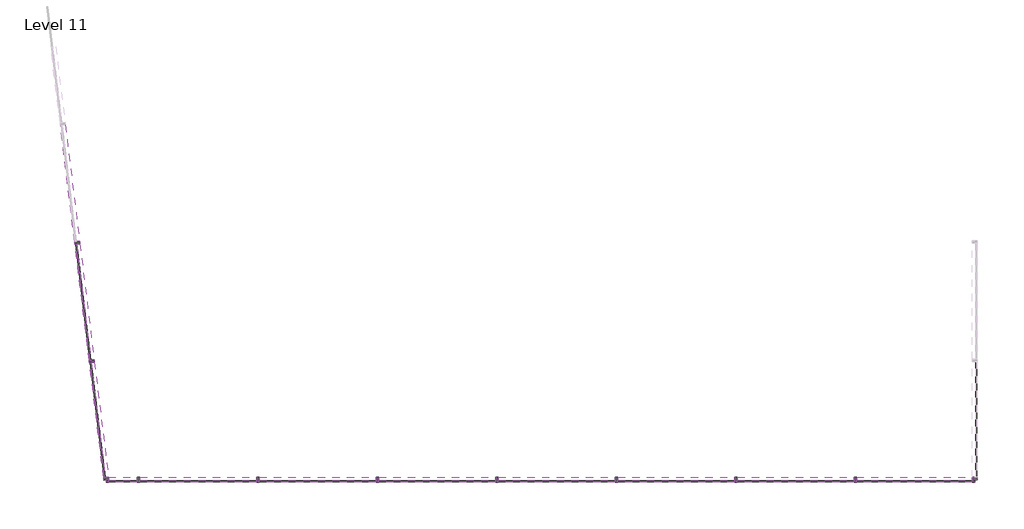
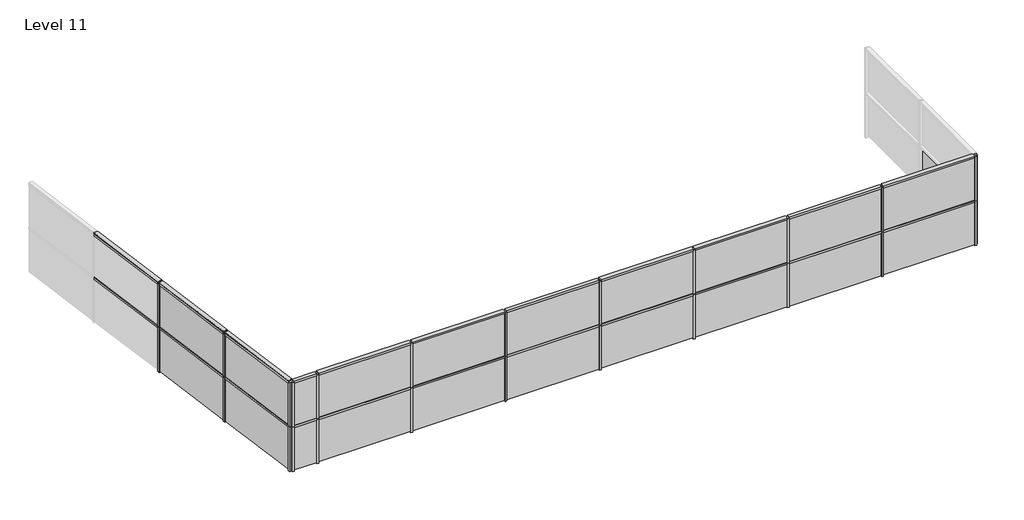
# One storey, part 1 of 2: 60 members, 25 plates.
"""IFC4 building model written with IfcOpenShell, lengths in millimetres."""

from ifc_helpers import new_model, si_unit, origin, place, context, project, spatial, transform, mapped, element, save
from components import member_daa7a266, member_82905deb, member_19d0a4ec, member_8cef0660, member_db480205, member_4491d118, member_0c11e56c, system_panel_glazed_37f15d2e, system_panel_glazed_3620f98e, system_panel_glazed_e46d4b42, system_panel_glazed_2a6c68b7, system_panel_glazed_9d0e0944

model = new_model("IFC4")

# Units and contexts
model_context = context("Model", 3, world=origin())
ifc_project = project(units=[si_unit("LENGTHUNIT", "METRE", prefix="MILLI")], contexts=[model_context])

# Site, building, storey
site = spatial("IfcSite", under=ifc_project)
building = spatial("IfcBuilding", under=site)
storey = spatial("IfcBuildingStorey", under=building, Name="Level 11", Elevation=30480.0)

# Members
placement = place(None, origin())
member_shape = member_daa7a266(model_context)
element("IfcMember", 1, ObjectType="Rectangular Mullion : 2.5\" x 5\" rectangular", at=placement, inside=storey, context=model_context, shape_type="MappedRepresentation", body=[
    mapped(member_shape, transform((-8260.4765148, -6916.1096898, 33528.0), x_axis=(0.0, 0.0, 1.0), y_axis=(-0.9925461516413222, -0.12186934340514587, 0.0), z_axis=(0.12186934340514587, -0.9925461516413222, 0.0))),
])
member_2_shape = member_82905deb(model_context)
element("IfcMember", 2, ObjectType="Rectangular Mullion : 2.5\" x 5\" rectangular", at=placement, inside=storey, context=model_context, shape_type="MappedRepresentation", body=[
    mapped(member_2_shape, transform((-8624.1955702, -3953.8557, 33528.0), x_axis=(-0.1218693434051459, 0.9925461516413222, 0.0), y_axis=(-0.9925461516413222, -0.1218693434051459, 0.0), z_axis=(0.0, 0.0, 1.0))),
])
element("IfcMember", 3, ObjectType="Rectangular Mullion : 2.5\" x 5\" rectangular", at=placement, inside=storey, context=model_context, shape_type="MappedRepresentation", body=[
    mapped(member_2_shape, transform((-8995.6533289, -928.5750297, 33528.0), x_axis=(-0.1218693434051459, 0.9925461516413222, 0.0), y_axis=(-0.9925461516413222, -0.1218693434051459, 0.0), z_axis=(0.0, 0.0, 1.0))),
])
member_3_shape = member_19d0a4ec(model_context)
element("IfcMember", 4, ObjectType="Rectangular Mullion : 2.5\" x 5\" rectangular", at=placement, inside=storey, context=model_context, shape_type="MappedRepresentation", body=[
    mapped(member_3_shape, transform((-8260.4765148, -6916.1096898, 32004.0), x_axis=(0.0, 0.0, 1.0), y_axis=(-0.9925461516413222, -0.12186934340514567, 0.0), z_axis=(0.12186934340514567, -0.9925461516413222, 0.0))),
])
element("IfcMember", 5, ObjectType="Rectangular Mullion : 2.5\" x 5\" rectangular", at=placement, inside=storey, context=model_context, shape_type="MappedRepresentation", body=[
    mapped(member_3_shape, transform((-8260.4765148, -6916.1096898, 32004.0), x_axis=(0.0, 0.0, 1.0), y_axis=(-0.9925461516413222, -0.12186934340514594, 0.0), z_axis=(0.12186934340514592, -0.9925461516413221, 0.0))),
])
element("IfcMember", 6, ObjectType="Rectangular Mullion : 2.5\" x 5\" rectangular", at=placement, inside=storey, context=model_context, shape_type="MappedRepresentation", body=[
    mapped(member_3_shape, transform((-8260.4765148, -6916.1096898, 33528.0), x_axis=(0.0, 0.0, 1.0), y_axis=(-0.9925461516413222, -0.12186934340514585, 0.0), z_axis=(0.12186934340514584, -0.9925461516413221, 0.0))),
])
element("IfcMember", 7, ObjectType="Rectangular Mullion : 2.5\" x 5\" rectangular", at=placement, inside=storey, context=model_context, shape_type="MappedRepresentation", body=[
    mapped(member_3_shape, transform((13839.0156363, -6979.1363705, 32004.0), x_axis=(0.0, 0.0, 1.0), y_axis=(0.0, -1.0, 0.0), z_axis=(1.0, 0.0, 0.0))),
])
element("IfcMember", 8, ObjectType="Rectangular Mullion : 2.5\" x 5\" rectangular", at=placement, inside=storey, context=model_context, shape_type="MappedRepresentation", body=[
    mapped(member_3_shape, transform((13839.0156363, -6979.1363705, 33528.0), x_axis=(0.0, 0.0, 1.0), y_axis=(0.0, -1.0, 0.0), z_axis=(1.0, 0.0, 0.0))),
])
member_4_shape = member_8cef0660(model_context)
element("IfcMember", 9, ObjectType="Rectangular Mullion : 2.5\" x 5\" rectangular", at=placement, inside=storey, context=model_context, shape_type="MappedRepresentation", body=[
    mapped(member_4_shape, transform((-8628.0649219, -3922.3423596, 32004.0), x_axis=(0.0, 0.0, 1.0), y_axis=(-0.9925461516413222, -0.12186934340514595, 0.0), z_axis=(0.12186934340514595, -0.9925461516413222, 0.0))),
])
element("IfcMember", 10, ObjectType="Rectangular Mullion : 2.5\" x 5\" rectangular", at=placement, inside=storey, context=model_context, shape_type="MappedRepresentation", body=[
    mapped(member_4_shape, transform((-8999.5226806, -897.0616894, 32004.0), x_axis=(0.0, 0.0, 1.0), y_axis=(-0.9925461516413222, -0.12186934340514599, 0.0), z_axis=(0.12186934340514599, -0.9925461516413222, 0.0))),
])
element("IfcMember", 11, ObjectType="Rectangular Mullion : 2.5\" x 5\" rectangular", at=placement, inside=storey, context=model_context, shape_type="MappedRepresentation", body=[
    mapped(member_4_shape, transform((-8628.0649219, -3922.3423596, 32004.0), x_axis=(0.0, 0.0, 1.0), y_axis=(-0.9925461516413222, -0.12186934340514607, 0.0), z_axis=(0.12186934340514607, -0.9925461516413222, 0.0))),
])
element("IfcMember", 12, ObjectType="Rectangular Mullion : 2.5\" x 5\" rectangular", at=placement, inside=storey, context=model_context, shape_type="MappedRepresentation", body=[
    mapped(member_4_shape, transform((-8999.5226806, -897.0616894, 32004.0), x_axis=(0.0, 0.0, 1.0), y_axis=(-0.9925461516413222, -0.12186934340514592, 0.0), z_axis=(0.12186934340514592, -0.9925461516413222, 0.0))),
])
element("IfcMember", 13, ObjectType="Rectangular Mullion : 2.5\" x 5\" rectangular", at=placement, inside=storey, context=model_context, shape_type="MappedRepresentation", body=[
    mapped(member_4_shape, transform((-8628.0649219, -3922.3423596, 33528.0), x_axis=(0.0, 0.0, 1.0), y_axis=(-0.9925461516413222, -0.1218693434051457, 0.0), z_axis=(0.1218693434051457, -0.9925461516413222, 0.0))),
])
element("IfcMember", 14, ObjectType="Rectangular Mullion : 2.5\" x 5\" rectangular", at=placement, inside=storey, context=model_context, shape_type="MappedRepresentation", body=[
    mapped(member_4_shape, transform((-8999.5226806, -897.0616894, 33528.0), x_axis=(0.0, 0.0, 1.0), y_axis=(-0.9925461516413222, -0.12186934340514595, 0.0), z_axis=(0.12186934340514595, -0.9925461516413222, 0.0))),
])
element("IfcMember", 15, ObjectType="Rectangular Mullion : 2.5\" x 5\" rectangular", at=placement, inside=storey, context=model_context, shape_type="MappedRepresentation", body=[
    mapped(member_4_shape, transform((10822.765636, -6979.1363705, 32004.0), x_axis=(0.0, 0.0, 1.0), y_axis=(0.0, -1.0, 0.0), z_axis=(1.0, 0.0, 0.0))),
])
element("IfcMember", 16, ObjectType="Rectangular Mullion : 2.5\" x 5\" rectangular", at=placement, inside=storey, context=model_context, shape_type="MappedRepresentation", body=[
    mapped(member_4_shape, transform((7774.765636, -6979.1363705, 32004.0), x_axis=(0.0, 0.0, 1.0), y_axis=(0.0, -1.0, 0.0), z_axis=(1.0, 0.0, 0.0))),
])
element("IfcMember", 17, ObjectType="Rectangular Mullion : 2.5\" x 5\" rectangular", at=placement, inside=storey, context=model_context, shape_type="MappedRepresentation", body=[
    mapped(member_4_shape, transform((4726.765636, -6979.1363705, 32004.0), x_axis=(0.0, 0.0, 1.0), y_axis=(0.0, -1.0, 0.0), z_axis=(1.0, 0.0, 0.0))),
])
element("IfcMember", 18, ObjectType="Rectangular Mullion : 2.5\" x 5\" rectangular", at=placement, inside=storey, context=model_context, shape_type="MappedRepresentation", body=[
    mapped(member_4_shape, transform((1678.765636, -6979.1363705, 32004.0), x_axis=(0.0, 0.0, 1.0), y_axis=(0.0, -1.0, 0.0), z_axis=(1.0, 0.0, 0.0))),
])
element("IfcMember", 19, ObjectType="Rectangular Mullion : 2.5\" x 5\" rectangular", at=placement, inside=storey, context=model_context, shape_type="MappedRepresentation", body=[
    mapped(member_4_shape, transform((-1369.234364, -6979.1363705, 32004.0), x_axis=(0.0, 0.0, 1.0), y_axis=(0.0, -1.0, 0.0), z_axis=(1.0, 0.0, 0.0))),
])
element("IfcMember", 20, ObjectType="Rectangular Mullion : 2.5\" x 5\" rectangular", at=placement, inside=storey, context=model_context, shape_type="MappedRepresentation", body=[
    mapped(member_4_shape, transform((-4417.234364, -6979.1363705, 32004.0), x_axis=(0.0, 0.0, 1.0), y_axis=(0.0, -1.0, 0.0), z_axis=(1.0, 0.0, 0.0))),
])
element("IfcMember", 21, ObjectType="Rectangular Mullion : 2.5\" x 5\" rectangular", at=placement, inside=storey, context=model_context, shape_type="MappedRepresentation", body=[
    mapped(member_4_shape, transform((10822.765636, -6979.1363705, 33528.0), x_axis=(0.0, 0.0, 1.0), y_axis=(0.0, -1.0, 0.0), z_axis=(1.0, 0.0, 0.0))),
])
element("IfcMember", 22, ObjectType="Rectangular Mullion : 2.5\" x 5\" rectangular", at=placement, inside=storey, context=model_context, shape_type="MappedRepresentation", body=[
    mapped(member_4_shape, transform((7774.765636, -6979.1363705, 33528.0), x_axis=(0.0, 0.0, 1.0), y_axis=(0.0, -1.0, 0.0), z_axis=(1.0, 0.0, 0.0))),
])
element("IfcMember", 23, ObjectType="Rectangular Mullion : 2.5\" x 5\" rectangular", at=placement, inside=storey, context=model_context, shape_type="MappedRepresentation", body=[
    mapped(member_4_shape, transform((4726.765636, -6979.1363705, 33528.0), x_axis=(0.0, 0.0, 1.0), y_axis=(0.0, -1.0, 0.0), z_axis=(1.0, 0.0, 0.0))),
])
element("IfcMember", 24, ObjectType="Rectangular Mullion : 2.5\" x 5\" rectangular", at=placement, inside=storey, context=model_context, shape_type="MappedRepresentation", body=[
    mapped(member_4_shape, transform((1678.765636, -6979.1363705, 33528.0), x_axis=(0.0, 0.0, 1.0), y_axis=(0.0, -1.0, 0.0), z_axis=(1.0, 0.0, 0.0))),
])
element("IfcMember", 25, ObjectType="Rectangular Mullion : 2.5\" x 5\" rectangular", at=placement, inside=storey, context=model_context, shape_type="MappedRepresentation", body=[
    mapped(member_4_shape, transform((-1369.234364, -6979.1363705, 33528.0), x_axis=(0.0, 0.0, 1.0), y_axis=(0.0, -1.0, 0.0), z_axis=(1.0, 0.0, 0.0))),
])
element("IfcMember", 26, ObjectType="Rectangular Mullion : 2.5\" x 5\" rectangular", at=placement, inside=storey, context=model_context, shape_type="MappedRepresentation", body=[
    mapped(member_4_shape, transform((-4417.234364, -6979.1363705, 33528.0), x_axis=(0.0, 0.0, 1.0), y_axis=(0.0, -1.0, 0.0), z_axis=(1.0, 0.0, 0.0))),
])
member_5_shape = member_db480205(model_context)
element("IfcMember", 27, ObjectType="Rectangular Mullion : 2.5\" x 5\" rectangular", at=placement, inside=storey, context=model_context, shape_type="MappedRepresentation", body=[
    mapped(member_5_shape, transform((-8628.0649219, -3922.3423596, 33528.0), x_axis=(0.0, 0.0, 1.0), y_axis=(-0.9925461516413222, -0.12186934340514592, 0.0), z_axis=(0.12186934340514592, -0.9925461516413222, 0.0))),
])
element("IfcMember", 28, ObjectType="Rectangular Mullion : 2.5\" x 5\" rectangular", at=placement, inside=storey, context=model_context, shape_type="MappedRepresentation", body=[
    mapped(member_5_shape, transform((-8999.5226806, -897.0616894, 33528.0), x_axis=(0.0, 0.0, 1.0), y_axis=(-0.9925461516413222, -0.12186934340514596, 0.0), z_axis=(0.12186934340514596, -0.9925461516413222, 0.0))),
])
element("IfcMember", 29, ObjectType="Rectangular Mullion : 2.5\" x 5\" rectangular", at=placement, inside=storey, context=model_context, shape_type="MappedRepresentation", body=[
    mapped(member_2_shape, transform((-8624.1955702, -3953.8557, 32004.0), x_axis=(-0.1218693434051459, 0.9925461516413222, 0.0), y_axis=(-0.9925461516413222, -0.1218693434051459, 0.0), z_axis=(0.0, 0.0, 1.0))),
])
element("IfcMember", 30, ObjectType="Rectangular Mullion : 2.5\" x 5\" rectangular", at=placement, inside=storey, context=model_context, shape_type="MappedRepresentation", body=[
    mapped(member_2_shape, transform((-8995.6533289, -928.5750297, 32004.0), x_axis=(-0.1218693434051459, 0.9925461516413222, 0.0), y_axis=(-0.9925461516413222, -0.1218693434051459, 0.0), z_axis=(0.0, 0.0, 1.0))),
])
element("IfcMember", 31, ObjectType="Rectangular Mullion : 2.5\" x 5\" rectangular", at=placement, inside=storey, context=model_context, shape_type="MappedRepresentation", body=[
    mapped(member_2_shape, transform((-8624.1955702, -3953.8557, 32004.0), x_axis=(-0.1218693434051459, 0.9925461516413222, 0.0), y_axis=(-0.9925461516413222, -0.1218693434051459, 0.0), z_axis=(0.0, 0.0, 1.0))),
])
element("IfcMember", 32, ObjectType="Rectangular Mullion : 2.5\" x 5\" rectangular", at=placement, inside=storey, context=model_context, shape_type="MappedRepresentation", body=[
    mapped(member_2_shape, transform((-8624.1955702, -3953.8557, 33528.0), x_axis=(-0.1218693434051459, 0.9925461516413222, 0.0), y_axis=(-0.9925461516413222, -0.1218693434051459, 0.0), z_axis=(0.0, 0.0, 1.0))),
])
element("IfcMember", 33, ObjectType="Rectangular Mullion : 2.5\" x 5\" rectangular", at=placement, inside=storey, context=model_context, shape_type="MappedRepresentation", body=[
    mapped(member_2_shape, transform((-8995.6533289, -928.5750297, 32004.0), x_axis=(-0.1218693434051459, 0.9925461516413222, 0.0), y_axis=(-0.9925461516413222, -0.1218693434051459, 0.0), z_axis=(0.0, 0.0, 1.0))),
])
element("IfcMember", 34, ObjectType="Rectangular Mullion : 2.5\" x 5\" rectangular", at=placement, inside=storey, context=model_context, shape_type="MappedRepresentation", body=[
    mapped(member_2_shape, transform((-8995.6533289, -928.5750297, 33528.0), x_axis=(-0.1218693434051459, 0.9925461516413222, 0.0), y_axis=(-0.9925461516413222, -0.1218693434051459, 0.0), z_axis=(0.0, 0.0, 1.0))),
])
element("IfcMember", 35, ObjectType="Rectangular Mullion : 2.5\" x 5\" rectangular", at=placement, inside=storey, context=model_context, shape_type="MappedRepresentation", body=[
    mapped(member_2_shape, transform((10854.515636, -6979.1363705, 32004.0), x_axis=(-1.0, 0.0, 0.0), y_axis=(0.0, -1.0, 0.0), z_axis=(0.0, 0.0, 1.0))),
])
element("IfcMember", 36, ObjectType="Rectangular Mullion : 2.5\" x 5\" rectangular", at=placement, inside=storey, context=model_context, shape_type="MappedRepresentation", body=[
    mapped(member_2_shape, transform((10854.515636, -6979.1363705, 33528.0), x_axis=(-1.0, 0.0, 0.0), y_axis=(0.0, -1.0, 0.0), z_axis=(0.0, 0.0, 1.0))),
])
element("IfcMember", 37, ObjectType="Rectangular Mullion : 2.5\" x 5\" rectangular", at=placement, inside=storey, context=model_context, shape_type="MappedRepresentation", body=[
    mapped(member_2_shape, transform((7806.515636, -6979.1363705, 32004.0), x_axis=(-1.0, 0.0, 0.0), y_axis=(0.0, -1.0, 0.0), z_axis=(0.0, 0.0, 1.0))),
])
element("IfcMember", 38, ObjectType="Rectangular Mullion : 2.5\" x 5\" rectangular", at=placement, inside=storey, context=model_context, shape_type="MappedRepresentation", body=[
    mapped(member_2_shape, transform((7806.515636, -6979.1363705, 33528.0), x_axis=(-1.0, 0.0, 0.0), y_axis=(0.0, -1.0, 0.0), z_axis=(0.0, 0.0, 1.0))),
])
element("IfcMember", 39, ObjectType="Rectangular Mullion : 2.5\" x 5\" rectangular", at=placement, inside=storey, context=model_context, shape_type="MappedRepresentation", body=[
    mapped(member_2_shape, transform((4758.515636, -6979.1363705, 32004.0), x_axis=(-1.0, 0.0, 0.0), y_axis=(0.0, -1.0, 0.0), z_axis=(0.0, 0.0, 1.0))),
])
element("IfcMember", 40, ObjectType="Rectangular Mullion : 2.5\" x 5\" rectangular", at=placement, inside=storey, context=model_context, shape_type="MappedRepresentation", body=[
    mapped(member_2_shape, transform((4758.515636, -6979.1363705, 33528.0), x_axis=(-1.0, 0.0, 0.0), y_axis=(0.0, -1.0, 0.0), z_axis=(0.0, 0.0, 1.0))),
])
element("IfcMember", 41, ObjectType="Rectangular Mullion : 2.5\" x 5\" rectangular", at=placement, inside=storey, context=model_context, shape_type="MappedRepresentation", body=[
    mapped(member_2_shape, transform((1710.515636, -6979.1363705, 32004.0), x_axis=(-1.0, 0.0, 0.0), y_axis=(0.0, -1.0, 0.0), z_axis=(0.0, 0.0, 1.0))),
])
element("IfcMember", 42, ObjectType="Rectangular Mullion : 2.5\" x 5\" rectangular", at=placement, inside=storey, context=model_context, shape_type="MappedRepresentation", body=[
    mapped(member_2_shape, transform((1710.515636, -6979.1363705, 33528.0), x_axis=(-1.0, 0.0, 0.0), y_axis=(0.0, -1.0, 0.0), z_axis=(0.0, 0.0, 1.0))),
])
element("IfcMember", 43, ObjectType="Rectangular Mullion : 2.5\" x 5\" rectangular", at=placement, inside=storey, context=model_context, shape_type="MappedRepresentation", body=[
    mapped(member_2_shape, transform((-1337.484364, -6979.1363705, 32004.0), x_axis=(-1.0, 0.0, 0.0), y_axis=(0.0, -1.0, 0.0), z_axis=(0.0, 0.0, 1.0))),
])
element("IfcMember", 44, ObjectType="Rectangular Mullion : 2.5\" x 5\" rectangular", at=placement, inside=storey, context=model_context, shape_type="MappedRepresentation", body=[
    mapped(member_2_shape, transform((-1337.484364, -6979.1363705, 33528.0), x_axis=(-1.0, 0.0, 0.0), y_axis=(0.0, -1.0, 0.0), z_axis=(0.0, 0.0, 1.0))),
])
element("IfcMember", 45, ObjectType="Rectangular Mullion : 2.5\" x 5\" rectangular", at=placement, inside=storey, context=model_context, shape_type="MappedRepresentation", body=[
    mapped(member_2_shape, transform((-4385.484364, -6979.1363705, 32004.0), x_axis=(-1.0, 0.0, 0.0), y_axis=(0.0, -1.0, 0.0), z_axis=(0.0, 0.0, 1.0))),
])
element("IfcMember", 46, ObjectType="Rectangular Mullion : 2.5\" x 5\" rectangular", at=placement, inside=storey, context=model_context, shape_type="MappedRepresentation", body=[
    mapped(member_2_shape, transform((-4385.484364, -6979.1363705, 33528.0), x_axis=(-1.0, 0.0, 0.0), y_axis=(0.0, -1.0, 0.0), z_axis=(0.0, 0.0, 1.0))),
])
element("IfcMember", 47, ObjectType="Rectangular Mullion : 2.5\" x 5\" rectangular", at=placement, inside=storey, context=model_context, shape_type="MappedRepresentation", body=[
    mapped(member_2_shape, transform((-7433.484364, -6979.1363705, 32004.0), x_axis=(-1.0, 0.0, 0.0), y_axis=(0.0, -1.0, 0.0), z_axis=(0.0, 0.0, 1.0))),
])
element("IfcMember", 48, ObjectType="Rectangular Mullion : 2.5\" x 5\" rectangular", at=placement, inside=storey, context=model_context, shape_type="MappedRepresentation", body=[
    mapped(member_2_shape, transform((-7433.484364, -6979.1363705, 33528.0), x_axis=(-1.0, 0.0, 0.0), y_axis=(0.0, -1.0, 0.0), z_axis=(0.0, 0.0, 1.0))),
])
member_6_shape = member_4491d118(model_context)
element("IfcMember", 49, ObjectType="Rectangular Mullion : 2.5\" x 5\" rectangular", at=placement, inside=storey, context=model_context, shape_type="MappedRepresentation", body=[
    mapped(member_6_shape, transform((-8252.7378115, -6979.1363705, 30480.0), x_axis=(0.1218693434051459, -0.9925461516413222, 0.0), y_axis=(-0.9925461516413222, -0.1218693434051459, 0.0), z_axis=(0.0, 0.0, -1.0))),
])
element("IfcMember", 50, ObjectType="Rectangular Mullion : 2.5\" x 5\" rectangular", at=placement, inside=storey, context=model_context, shape_type="MappedRepresentation", body=[
    mapped(member_6_shape, transform((-8252.7378115, -6979.1363705, 30480.0), x_axis=(0.1218693434051459, -0.9925461516413222, 0.0), y_axis=(-0.9925461516413222, -0.1218693434051459, 0.0), z_axis=(0.0, 0.0, -1.0))),
])
element("IfcMember", 51, ObjectType="Rectangular Mullion : 2.5\" x 5\" rectangular", at=placement, inside=storey, context=model_context, shape_type="MappedRepresentation", body=[
    mapped(member_6_shape, transform((-8252.7378115, -6979.1363705, 32004.0), x_axis=(0.1218693434051459, -0.9925461516413222, 0.0), y_axis=(-0.9925461516413222, -0.1218693434051459, 0.0), z_axis=(0.0, 0.0, -1.0))),
])
element("IfcMember", 52, ObjectType="Rectangular Mullion : 2.5\" x 5\" rectangular", at=placement, inside=storey, context=model_context, shape_type="MappedRepresentation", body=[
    mapped(member_6_shape, transform((13902.5156363, -6979.1363705, 30480.0), x_axis=(1.0, 0.0, 0.0), y_axis=(0.0, -1.0, 0.0), z_axis=(0.0, 0.0, -1.0))),
])
element("IfcMember", 53, ObjectType="Rectangular Mullion : 2.5\" x 5\" rectangular", at=placement, inside=storey, context=model_context, shape_type="MappedRepresentation", body=[
    mapped(member_6_shape, transform((13902.5156363, -6979.1363705, 32004.0), x_axis=(1.0, 0.0, 0.0), y_axis=(0.0, -1.0, 0.0), z_axis=(0.0, 0.0, -1.0))),
])
element("IfcMember", 54, ObjectType="Rectangular Mullion : 2.5\" x 5\" rectangular", at=placement, inside=storey, context=model_context, shape_type="MappedRepresentation", body=[
    mapped(member_6_shape, transform((-8252.7378115, -6979.1363705, 32004.0), x_axis=(0.1218693434051459, -0.9925461516413222, 0.0), y_axis=(-0.9925461516413222, -0.1218693434051459, 0.0), z_axis=(0.0, 0.0, -1.0))),
])
element("IfcMember", 55, ObjectType="Rectangular Mullion : 2.5\" x 5\" rectangular", at=placement, inside=storey, context=model_context, shape_type="MappedRepresentation", body=[
    mapped(member_6_shape, transform((-8252.7378115, -6979.1363705, 32004.0), x_axis=(-1.0, 0.0, 0.0), y_axis=(0.0, -1.0, 0.0), z_axis=(0.0, 0.0, 1.0))),
])
element("IfcMember", 56, ObjectType="Rectangular Mullion : 2.5\" x 5\" rectangular", at=placement, inside=storey, context=model_context, shape_type="MappedRepresentation", body=[
    mapped(member_6_shape, transform((-8252.7378115, -6979.1363705, 33528.0), x_axis=(-1.0, 0.0, 0.0), y_axis=(0.0, -1.0, 0.0), z_axis=(0.0, 0.0, 1.0))),
])
element("IfcMember", 57, ObjectType="Rectangular Mullion : 2.5\" x 5\" rectangular", at=placement, inside=storey, context=model_context, shape_type="MappedRepresentation", body=[
    mapped(member_6_shape, transform((13902.5156363, -6979.1363705, 32004.0), x_axis=(0.0, -1.0, 0.0), y_axis=(1.0, 0.0, 0.0), z_axis=(0.0, 0.0, 1.0))),
])
element("IfcMember", 58, ObjectType="Rectangular Mullion : 2.5\" x 5\" rectangular", at=placement, inside=storey, context=model_context, shape_type="MappedRepresentation", body=[
    mapped(member_6_shape, transform((13902.5156363, -6979.1363705, 33528.0), x_axis=(0.0, -1.0, 0.0), y_axis=(1.0, 0.0, 0.0), z_axis=(0.0, 0.0, 1.0))),
])
member_7_shape = member_0c11e56c(model_context)
element("IfcMember", 59, ObjectType="Rectangular Mullion : 2.5\" x 5\" rectangular", at=placement, inside=storey, context=model_context, shape_type="MappedRepresentation", body=[
    mapped(member_7_shape, transform((-7465.234364, -6979.1363705, 32004.0), x_axis=(0.0, 0.0, 1.0), y_axis=(0.0, -1.0, 0.0), z_axis=(1.0, 0.0, 0.0))),
])
element("IfcMember", 60, ObjectType="Rectangular Mullion : 2.5\" x 5\" rectangular", at=placement, inside=storey, context=model_context, shape_type="MappedRepresentation", body=[
    mapped(member_7_shape, transform((-7465.234364, -6979.1363705, 33528.0), x_axis=(0.0, 0.0, 1.0), y_axis=(0.0, -1.0, 0.0), z_axis=(1.0, 0.0, 0.0))),
])

# Plates
system_panel_glazed_shape = system_panel_glazed_37f15d2e(model_context)
element("IfcPlate", 61, ObjectType="System Panel : Glazed", at=placement, inside=storey, context=model_context, shape_type="MappedRepresentation", body=[
    mapped(system_panel_glazed_shape, transform((-8440.4013667, -5450.739365, 32035.75), x_axis=(-0.1218693434051459, 0.9925461516413222, 0.0), y_axis=(-0.9925461516413222, -0.1218693434051459, 0.0), z_axis=(0.0, 0.0, 1.0))),
])
system_panel_glazed_2_shape = system_panel_glazed_3620f98e(model_context)
element("IfcPlate", 62, ObjectType="System Panel : Glazed", at=placement, inside=storey, context=model_context, shape_type="MappedRepresentation", body=[
    mapped(system_panel_glazed_2_shape, transform((-8809.9244496, -2441.2153649, 32035.75), x_axis=(-0.1218693434051459, 0.9925461516413222, 0.0), y_axis=(-0.9925461516413222, -0.1218693434051459, 0.0), z_axis=(0.0, 0.0, 1.0))),
])
system_panel_glazed_3_shape = system_panel_glazed_e46d4b42(model_context)
element("IfcPlate", 63, ObjectType="System Panel : Glazed", at=placement, inside=storey, context=model_context, shape_type="MappedRepresentation", body=[
    mapped(system_panel_glazed_3_shape, transform((-8440.4013667, -5450.739365, 30511.75), x_axis=(-0.1218693434051459, 0.9925461516413222, 0.0), y_axis=(-0.9925461516413222, -0.1218693434051459, 0.0), z_axis=(0.0, 0.0, 1.0))),
])
element("IfcPlate", 64, ObjectType="System Panel : Glazed", at=placement, inside=storey, context=model_context, shape_type="MappedRepresentation", body=[
    mapped(system_panel_glazed_3_shape, transform((-8440.4013667, -5450.739365, 30511.75), x_axis=(-0.1218693434051459, 0.9925461516413222, 0.0), y_axis=(-0.9925461516413222, -0.1218693434051459, 0.0), z_axis=(0.0, 0.0, 1.0))),
])
element("IfcPlate", 65, ObjectType="System Panel : Glazed", at=placement, inside=storey, context=model_context, shape_type="MappedRepresentation", body=[
    mapped(system_panel_glazed_3_shape, transform((-8440.4013667, -5450.739365, 32035.75), x_axis=(-0.1218693434051459, 0.9925461516413222, 0.0), y_axis=(-0.9925461516413222, -0.1218693434051459, 0.0), z_axis=(0.0, 0.0, 1.0))),
])
element("IfcPlate", 66, ObjectType="System Panel : Glazed", at=placement, inside=storey, context=model_context, shape_type="MappedRepresentation", body=[
    mapped(system_panel_glazed_3_shape, transform((12362.6406361, -6979.1363705, 30511.75), x_axis=(-1.0, 0.0, 0.0), y_axis=(0.0, -1.0, 0.0), z_axis=(0.0, 0.0, 1.0))),
])
element("IfcPlate", 67, ObjectType="System Panel : Glazed", at=placement, inside=storey, context=model_context, shape_type="MappedRepresentation", body=[
    mapped(system_panel_glazed_3_shape, transform((12362.6406361, -6979.1363705, 32035.75), x_axis=(-1.0, 0.0, 0.0), y_axis=(0.0, -1.0, 0.0), z_axis=(0.0, 0.0, 1.0))),
])
element("IfcPlate", 68, ObjectType="System Panel : Glazed", at=placement, inside=storey, context=model_context, shape_type="MappedRepresentation", body=[
    mapped(system_panel_glazed_3_shape, transform((13902.5156363, -5439.2613706, 30511.75), x_axis=(0.0, -1.0, 0.0), y_axis=(1.0, 0.0, 0.0), z_axis=(0.0, 0.0, 1.0))),
])
system_panel_glazed_4_shape = system_panel_glazed_2a6c68b7(model_context)
element("IfcPlate", 69, ObjectType="System Panel : Glazed", at=placement, inside=storey, context=model_context, shape_type="MappedRepresentation", body=[
    mapped(system_panel_glazed_4_shape, transform((-8809.9244496, -2441.2153649, 30511.75), x_axis=(-0.1218693434051459, 0.9925461516413222, 0.0), y_axis=(-0.9925461516413222, -0.1218693434051459, 0.0), z_axis=(0.0, 0.0, 1.0))),
])
element("IfcPlate", 70, ObjectType="System Panel : Glazed", at=placement, inside=storey, context=model_context, shape_type="MappedRepresentation", body=[
    mapped(system_panel_glazed_4_shape, transform((-8809.9244496, -2441.2153649, 30511.75), x_axis=(-0.1218693434051459, 0.9925461516413222, 0.0), y_axis=(-0.9925461516413222, -0.1218693434051459, 0.0), z_axis=(0.0, 0.0, 1.0))),
])
element("IfcPlate", 71, ObjectType="System Panel : Glazed", at=placement, inside=storey, context=model_context, shape_type="MappedRepresentation", body=[
    mapped(system_panel_glazed_4_shape, transform((-8809.9244496, -2441.2153649, 32035.75), x_axis=(-0.1218693434051459, 0.9925461516413222, 0.0), y_axis=(-0.9925461516413222, -0.1218693434051459, 0.0), z_axis=(0.0, 0.0, 1.0))),
])
element("IfcPlate", 72, ObjectType="System Panel : Glazed", at=placement, inside=storey, context=model_context, shape_type="MappedRepresentation", body=[
    mapped(system_panel_glazed_4_shape, transform((9330.515636, -6979.1363705, 30511.75), x_axis=(-1.0, 0.0, 0.0), y_axis=(0.0, -1.0, 0.0), z_axis=(0.0, 0.0, 1.0))),
])
element("IfcPlate", 73, ObjectType="System Panel : Glazed", at=placement, inside=storey, context=model_context, shape_type="MappedRepresentation", body=[
    mapped(system_panel_glazed_4_shape, transform((6282.515636, -6979.1363705, 30511.75), x_axis=(-1.0, 0.0, 0.0), y_axis=(0.0, -1.0, 0.0), z_axis=(0.0, 0.0, 1.0))),
])
element("IfcPlate", 74, ObjectType="System Panel : Glazed", at=placement, inside=storey, context=model_context, shape_type="MappedRepresentation", body=[
    mapped(system_panel_glazed_4_shape, transform((3234.515636, -6979.1363705, 30511.75), x_axis=(-1.0, 0.0, 0.0), y_axis=(0.0, -1.0, 0.0), z_axis=(0.0, 0.0, 1.0))),
])
element("IfcPlate", 75, ObjectType="System Panel : Glazed", at=placement, inside=storey, context=model_context, shape_type="MappedRepresentation", body=[
    mapped(system_panel_glazed_4_shape, transform((186.515636, -6979.1363705, 30511.75), x_axis=(-1.0, 0.0, 0.0), y_axis=(0.0, -1.0, 0.0), z_axis=(0.0, 0.0, 1.0))),
])
element("IfcPlate", 76, ObjectType="System Panel : Glazed", at=placement, inside=storey, context=model_context, shape_type="MappedRepresentation", body=[
    mapped(system_panel_glazed_4_shape, transform((-2861.484364, -6979.1363705, 30511.75), x_axis=(-1.0, 0.0, 0.0), y_axis=(0.0, -1.0, 0.0), z_axis=(0.0, 0.0, 1.0))),
])
element("IfcPlate", 77, ObjectType="System Panel : Glazed", at=placement, inside=storey, context=model_context, shape_type="MappedRepresentation", body=[
    mapped(system_panel_glazed_4_shape, transform((-5909.484364, -6979.1363705, 30511.75), x_axis=(-1.0, 0.0, 0.0), y_axis=(0.0, -1.0, 0.0), z_axis=(0.0, 0.0, 1.0))),
])
element("IfcPlate", 78, ObjectType="System Panel : Glazed", at=placement, inside=storey, context=model_context, shape_type="MappedRepresentation", body=[
    mapped(system_panel_glazed_4_shape, transform((9330.515636, -6979.1363705, 32035.75), x_axis=(-1.0, 0.0, 0.0), y_axis=(0.0, -1.0, 0.0), z_axis=(0.0, 0.0, 1.0))),
])
element("IfcPlate", 79, ObjectType="System Panel : Glazed", at=placement, inside=storey, context=model_context, shape_type="MappedRepresentation", body=[
    mapped(system_panel_glazed_4_shape, transform((6282.515636, -6979.1363705, 32035.75), x_axis=(-1.0, 0.0, 0.0), y_axis=(0.0, -1.0, 0.0), z_axis=(0.0, 0.0, 1.0))),
])
element("IfcPlate", 80, ObjectType="System Panel : Glazed", at=placement, inside=storey, context=model_context, shape_type="MappedRepresentation", body=[
    mapped(system_panel_glazed_4_shape, transform((3234.515636, -6979.1363705, 32035.75), x_axis=(-1.0, 0.0, 0.0), y_axis=(0.0, -1.0, 0.0), z_axis=(0.0, 0.0, 1.0))),
])
element("IfcPlate", 81, ObjectType="System Panel : Glazed", at=placement, inside=storey, context=model_context, shape_type="MappedRepresentation", body=[
    mapped(system_panel_glazed_4_shape, transform((186.515636, -6979.1363705, 32035.75), x_axis=(-1.0, 0.0, 0.0), y_axis=(0.0, -1.0, 0.0), z_axis=(0.0, 0.0, 1.0))),
])
element("IfcPlate", 82, ObjectType="System Panel : Glazed", at=placement, inside=storey, context=model_context, shape_type="MappedRepresentation", body=[
    mapped(system_panel_glazed_4_shape, transform((-2861.484364, -6979.1363705, 32035.75), x_axis=(-1.0, 0.0, 0.0), y_axis=(0.0, -1.0, 0.0), z_axis=(0.0, 0.0, 1.0))),
])
element("IfcPlate", 83, ObjectType="System Panel : Glazed", at=placement, inside=storey, context=model_context, shape_type="MappedRepresentation", body=[
    mapped(system_panel_glazed_4_shape, transform((-5909.484364, -6979.1363705, 32035.75), x_axis=(-1.0, 0.0, 0.0), y_axis=(0.0, -1.0, 0.0), z_axis=(0.0, 0.0, 1.0))),
])
system_panel_glazed_5_shape = system_panel_glazed_9d0e0944(model_context)
element("IfcPlate", 84, ObjectType="System Panel : Glazed", at=placement, inside=storey, context=model_context, shape_type="MappedRepresentation", body=[
    mapped(system_panel_glazed_5_shape, transform((-7827.2360878, -6979.1363705, 30511.75), x_axis=(-1.0, 0.0, 0.0), y_axis=(0.0, -1.0, 0.0), z_axis=(0.0, 0.0, 1.0))),
])
element("IfcPlate", 85, ObjectType="System Panel : Glazed", at=placement, inside=storey, context=model_context, shape_type="MappedRepresentation", body=[
    mapped(system_panel_glazed_5_shape, transform((-7827.2360878, -6979.1363705, 32035.75), x_axis=(-1.0, 0.0, 0.0), y_axis=(0.0, -1.0, 0.0), z_axis=(0.0, 0.0, 1.0))),
])

save(model, "model.ifc")

# Revit data of these elements
# Type "Rectangular Mullion : 2.5\" x 5\" rectangular"
#   built-in parameter 1007304 = 0.416667 (stored number, unit not read)
#   built-in parameter 1007301 = 0.104167 (stored number, unit not read)
#   built-in parameter 1007300 = 0.104167 (stored number, unit not read)
# Type "System Panel : Glazed"
#   Construction Type Id = "GSP4R"
#   Analytic Construction = "1/8 in Pilkington single glazing"
#   Visual Light Transmittance = 0.9
#   Solar Heat Gain Coefficient = 0.86
#   Heat Transfer Coefficient (U) = 1.18115 BTU/(h·ft²·°F)
#   Define Thermal Properties by = 1
# Elements 1, 2, 3, 4, 5, 6, 7, 8, 9, 10, 11, 12, 13, 14, 15, 16, 17, 18, 19, 20, 21, 22, 23, 24, 25, 26, 27, 28, 29, 30, 31, 32, 33, 34, 35, 36, 37, 38, 39, 40, 41, 42, 43, 44, 45, 46, 47, 48, 49, 50, 51, 52, 53, 54, 55, 56, 57, 58, 59, 60 (IfcMember, "Rectangular Mullion : 2.5\" x 5\" rectangular")
#   Phase Created = New Construction
#   Materials on its faces: "Aluminum"
# Elements 61, 62, 63, 64, 65, 66, 67, 68, 69, 70, 71, 72, 73, 74, 75, 76, 77, 78, 79, 80, 81, 82, 83, 84, 85 (IfcPlate, "System Panel : Glazed")
#   Phase Created = New Construction
#   Materials on its faces: "Glass"
# Materials
#   "Aluminum": class "Metal", colour RGB 247 247 247, transparency 0, Description = "Aluminum 6061", Cost = 0
#   "Glass": class "Glass", colour RGB 0 128 192, transparency 0.75, Description = "Soda Lime Glass", Cost = 0
